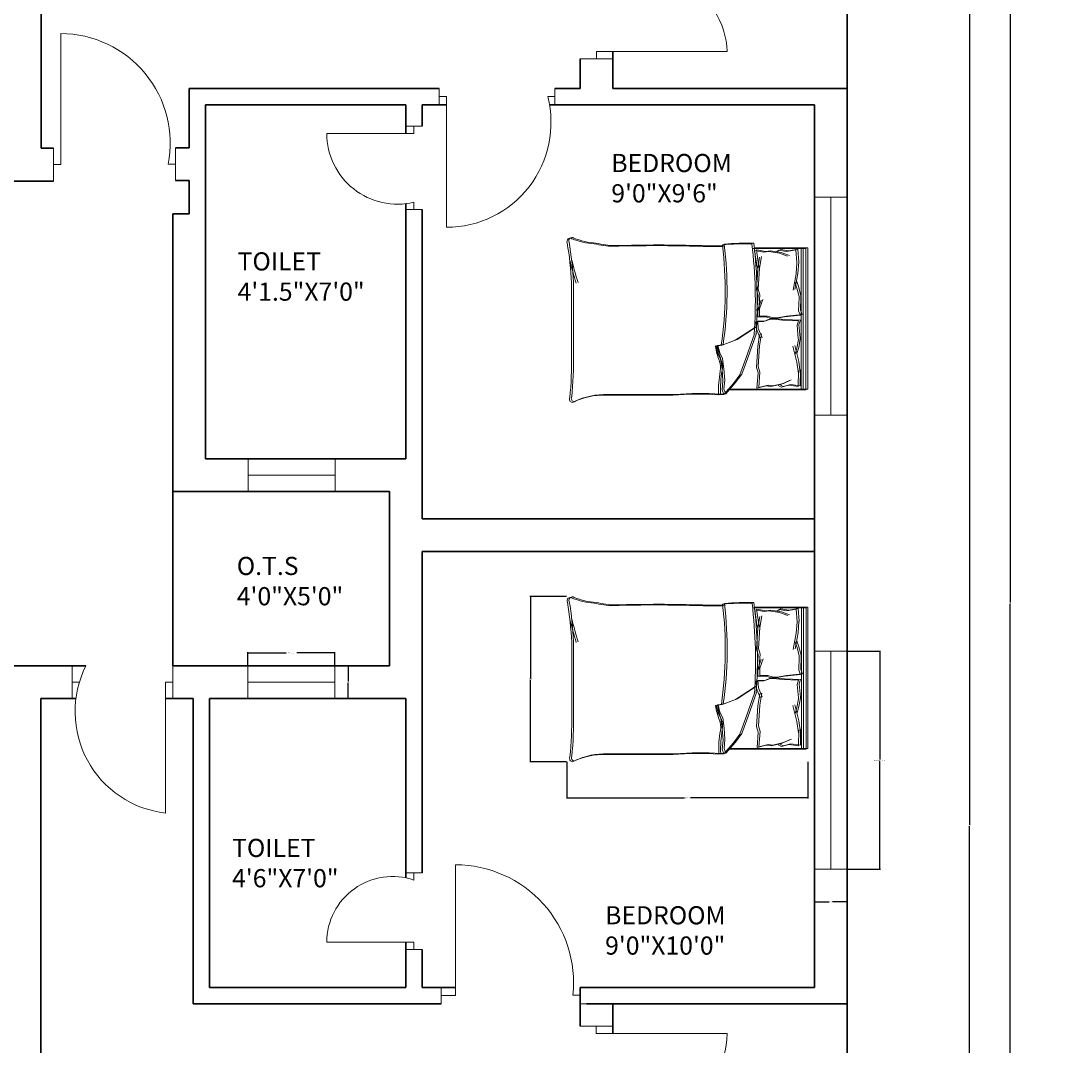
# Model space of a CAD drawing. Units: inches. Extents: x 2250 to 3629, y 982 to 2740.
# Tile 4 of 12: x 2629 to 2918, y 1543 to 1825. Entities that reach past the tile are written whole.
import ezdxf

# ---------------------------------------------------------------- set-up
doc = ezdxf.new("R2010")
doc.units = ezdxf.units.IN
for name, color, linetype, lineweight in [('A-ANNO-DIMS', 2, 'Continuous', 18), ('A-AREA-IDEN', 7, 'Continuous', 18), ('A-DOOR', 3, 'Continuous', 18), ('A-FURN', 8, 'Continuous', 13), ('A-GLAZ', 4, 'Continuous', 18), ('A-WALL', 7, 'Continuous', 35)]:
    doc.layers.add(name, color=color, linetype=linetype, lineweight=lineweight)
doc.styles.get("Standard").update_dxf_attribs({"font": 'arial.ttf'})
doc.dimstyles.get("Standard").update_dxf_attribs({"dimtxt": 0.18, "dimasz": 0.18, "dimexe": 0.18, "dimexo": 0.0625, "dimgap": 0.09, "dimtad": 0, "dimtih": 1, "dimtoh": 1, "dimdec": 4, "dimzin": 0, "dimdsep": 46, "dimtxsty": 'Standard', "dimcen": 0.09, "dimadec": 0, "dimazin": 0, "dimtfac": 1, "dimtdec": 4, "dimtofl": 0, "dimtmove": 0, "dimatfit": 3, "dimfxl": 1, "dimtolj": 1, "dimtzin": 0, "dimarcsym": 0})

# ---------------------------------------------------------------- blocks, each defined once
blk = doc.blocks.new('DR-36-BED-EAST-N')
for p, q in [((0, 38.25), (0, 33.75)), ((31.87, 33.75), (31.87, 38.25)), ((31.87, 38.25), (31.87, 36)), ((0, 33.75), (0, 36)), ((0, 36), (2, 36)), ((2, 36), (2, 0)), ((31.87, 36), (29.87, 36))]:
    blk.add_line(p, q)
blk.add_arc((2, 28.78), 28.78, 270, 14.5177)
blk = doc.blocks.new('DR-72-DECK-EAST-N')
for p, q in [((9, 42.6), (0, 42.6)), ((0, 42.6), (4.5, 42.6)), ((4.5, 42.6), (4.5, 40.6)), ((4.5, 40.6), (40.5, 40.6)), ((9, 0), (0, 0)), ((0, 0), (4.5, 0)), ((4.5, 0), (4.5, 2)), ((4.5, 2), (40.5, 2))]:
    blk.add_line(p, q)
for centre, radius, start, end in [((18.63, 40.6), 21.87, 295.9981, 0), ((18.59, 1.24), 21.93, 1.9829, 63.9515)]:
    blk.add_arc(centre, radius, start, end)
blk = doc.blocks.new('DR-36-BED-EAST-S')
for p, q in [((4, 2.25), (4, 38.25)), ((0, 4.5), (0, 0)), ((0, 0), (0, 2.25)), ((0, 2.25), (2, 2.25)), ((2, 2.25), (4, 2.25)), ((38.26, 2.37), (36.26, 2.37)), ((40.06, 0), (38.26, 0))]:
    blk.add_line(p, q)
blk.add_arc((4, 5.8), 32.45, 353.93, 90)
blk = doc.blocks.new('DR-72-DECK-EAST-S')
for p, q in [((5.33, 41.58), (0, 41.58)), ((0, 41.58), (4.45, 41.58)), ((9, 41.58), (1.67, 41.58)), ((1.67, 41.58), (5.33, 41.58)), ((4.45, 41.58), (4.45, 39.58)), ((4.45, 39.58), (40.45, 39.58)), ((4.5, 0), (4.5, 2)), ((4.5, 2), (40.5, 2)), ((9, 0), (0, 0)), ((0, 0), (4.5, 0))]:
    blk.add_line(p, q)
for centre, radius, start, end in [((18.64, 39.58), 21.82, 293.079, 0), ((16.02, -2.8), 24.94, 11.0871, 63.4091)]:
    blk.add_arc(centre, radius, start, end)
blk = doc.blocks.new('DR-24-BATH-EAST-S')
for p, q in [((21.75, 21.12), (26.25, 21.12)), ((26.25, 21.12), (24, 21.12)), ((24, 21.12), (24, 19.12)), ((24, 2), (0, 2)), ((24, 0), (24, 2)), ((26.25, 0), (21.75, 0)), ((21.75, 0), (24, 0))]:
    blk.add_line(p, q)
blk.add_arc((18.1, 2), 18.1, 70.988, 180)
blk = doc.blocks.new('DR-36-ENTRY-SE')
for p, q in [((0, 31.5), (0, 40.5)), ((27.72, 40.5), (27.72, 31.5)), ((0, 36), (2, 36)), ((27.72, 36), (25.72, 36)), ((25.72, 36), (25.72, 0)), ((27.72, 31.5), (27.72, 36))]:
    blk.add_line(p, q)
blk.add_arc((28.88, 27.9), 28.08, 153.3297, 263.5366)
blk = doc.blocks.new('DR-24-BATH-EAST-N')
for p, q in [((24, 20.95), (0, 20.95)), ((26.25, 22.95), (21.75, 22.95)), ((21.75, 22.95), (24, 22.95)), ((24, 22.95), (24, 20.95)), ((24, 0), (24, 2)), ((21.75, 0), (26.25, 0)), ((26.25, 0), (24, 0))]:
    blk.add_line(p, q)
blk.add_arc((19.48, 20.95), 19.48, 180, 283.4076)
blk = doc.blocks.new('DR-36-ENTRY-NE')
for p, q in [((2, 4.58), (2, 40.58)), ((0, 9), (0, 0)), ((33.56, 9.15), (33.56, 0.15)), ((0, 4.58), (2, 4.58)), ((33.56, 4.65), (31.56, 4.65))]:
    blk.add_line(p, q)
blk.add_arc((2, 10.45), 30.13, 348.9073, 90)
blk = doc.blocks.new('WIN-24-BATH-NW')
for p, q in [((9, 24), (0, 24)), ((0, 24), (4.5, 24)), ((4.5, 24), (4.5, 0)), ((9, 0), (0, 0)), ((4.5, 0), (9, 0))]:
    blk.add_line(p, q)
blk = doc.blocks.new('WIN-60-BED-EAST-S')
for p, q in [((0, 60), (9, 60)), ((9, 60), (4.5, 60)), ((4.5, 60), (4.5, 0)), ((9, 0), (0, 0)), ((4.5, 0), (9, 0))]:
    blk.add_line(p, q)
blk = doc.blocks.new('BED-WITH-PILLOWS')
for p, q in [((2.83, 51.56), (2.83, 66.3)), ((2.83, 66.3), (41.74, 66.3)), ((2.83, 65.05), (41.74, 65.05)), ((3.02, 51.04), (3.02, 65.78)), ((3.02, 65.78), (41.92, 65.78)), ((3.02, 64.53), (41.92, 64.53)), ((3.17, 63.59), (6.66, 63.85)), ((6.66, 63.85), (6.75, 63.84)), ((6.75, 63.84), (9.86, 63.6)), ((12.09, 63.25), (13.74, 63.84)), ((13.74, 63.84), (16.09, 64.43)), ((13.93, 63.32), (16.28, 63.91)), ((16.09, 64.43), (16.36, 64.43)), ((16.28, 63.91), (16.54, 63.91)), ((16.36, 64.43), (19.98, 64.31)), ((16.54, 63.91), (20.16, 63.79)), ((19.98, 64.31), (21.15, 64.78)), ((20.16, 63.79), (21.34, 64.26)), ((21.15, 64.78), (21.62, 60.43)), ((21.34, 64.26), (21.81, 59.9)), ((22.78, 64.27), (22.58, 59.9)), ((22.96, 63.75), (22.76, 59.38)), ((23.98, 63.88), (22.78, 64.27)), ((24.17, 63.36), (22.96, 63.75)), ((27.59, 64.22), (23.98, 63.88)), ((27.77, 63.7), (24.17, 63.36)), ((27.85, 64.24), (27.59, 64.22)), ((28.03, 63.72), (27.77, 63.7)), ((30.23, 63.8), (27.85, 64.24)), ((30.42, 63.28), (28.03, 63.72)), ((34.12, 63.8), (29.71, 62.7)), ((31.91, 63.31), (30.23, 63.8)), ((37.22, 64.23), (34.12, 63.8)), ((37.4, 63.71), (34.31, 63.28)), ((40.8, 64.22), (36.4, 64.3)), ((36.4, 64.3), (37.22, 64.23)), ((40.98, 63.7), (36.58, 63.78)), ((36.58, 63.78), (37.4, 63.71)), ((40.8, 64.22), (40.49, 61.61)), ((40.98, 63.7), (40.67, 61.09)), ((41.74, 66.3), (41.74, 44.64)), ((41.92, 65.78), (41.92, 44.12)), ((3.17, 63.6), (3.64, 61.01)), ((3.64, 61.01), (3.29, 58.89)), ((3.36, 63.06), (6.85, 63.33)), ((3.36, 63.08), (3.83, 60.49)), ((4.11, 59.01), (4.94, 61.25)), ((4.3, 58.49), (5.12, 60.73)), ((6.85, 63.33), (6.93, 63.32)), ((6.93, 63.32), (10.04, 63.08)), ((9.86, 63.6), (14.33, 62.78)), ((10.04, 63.08), (14.52, 62.26)), ((12.28, 62.73), (13.93, 63.32)), ((34.31, 63.28), (29.9, 62.18)), ((32.1, 62.79), (30.42, 63.28)), ((40.14, 59.58), (39.18, 61.76)), ((40.33, 59.06), (39.37, 61.24)), ((40.49, 61.61), (40.97, 59.51)), ((40.67, 61.09), (41.16, 58.99)), ((3.29, 58.89), (3.76, 58.07)), ((3.83, 60.49), (3.47, 58.37)), ((3.47, 58.37), (3.95, 57.55)), ((3.64, 56.07), (4.11, 59.01)), ((3.83, 55.55), (4.3, 58.49)), ((21.62, 60.43), (22.09, 57.84)), ((21.81, 59.9), (22.28, 57.32)), ((22.09, 57.84), (22.09, 56.78)), ((22.58, 59.9), (22.27, 57.28)), ((22.76, 59.38), (22.46, 56.76)), ((40.8, 56.67), (40.14, 59.58)), ((40.98, 56.15), (40.33, 59.06)), ((40.97, 59.51), (40.55, 58.66)), ((41.16, 58.99), (40.74, 58.14)), ((3.88, 54.78), (3.64, 56.07)), ((4.06, 54.25), (3.83, 55.55)), ((22.09, 56.78), (21.62, 55.25)), ((21.62, 55.25), (21.62, 53.06)), ((22.28, 56.26), (21.81, 54.73)), ((22.27, 57.28), (22.34, 56.23)), ((22.28, 57.32), (22.28, 56.26)), ((22.34, 56.23), (22.9, 54.73)), ((22.46, 56.76), (22.52, 55.71)), ((22.52, 55.71), (23.09, 54.21)), ((40.64, 55.37), (40.8, 56.67)), ((41.27, 52.81), (40.64, 55.37)), ((40.83, 54.85), (40.98, 56.15)), ((3.41, 52.19), (3.88, 54.78)), ((7.56, 52.77), (3.41, 52.19)), ((3.59, 51.66), (4.06, 54.25)), ((7.74, 52.25), (3.59, 51.66)), ((5.2, 53.58), (8.48, 53.04)), ((5.38, 53.06), (8.66, 52.52)), ((8.48, 53.04), (7.56, 52.77)), ((8.66, 52.52), (7.74, 52.25)), ((8.48, 53.04), (14.18, 52.69)), ((8.66, 52.52), (14.37, 52.17)), ((14.18, 52.69), (15.78, 53.14)), ((14.37, 52.17), (15.97, 52.62)), ((15.78, 53.14), (19.96, 52.81)), ((15.97, 52.62), (20.14, 52.29)), ((19.62, 53.06), (17.06, 53.95)), ((19.81, 52.54), (17.25, 53.43)), ((21.62, 53.06), (19.62, 53.06)), ((21.81, 52.54), (19.81, 52.54)), ((21.81, 54.73), (21.81, 52.54)), ((22.9, 54.73), (23.04, 52.55)), ((23.04, 52.55), (25.03, 52.68)), ((23.09, 54.21), (23.22, 52.03)), ((23.22, 52.03), (25.22, 52.15)), ((24.63, 52.15), (28.05, 46.86)), ((25.03, 52.68), (27.53, 53.72)), ((25.22, 52.15), (27.72, 53.2)), ((33.09, 49.76), (26.3, 52.15)), ((26.51, 53.58), (29.79, 53.04)), ((26.7, 53.06), (29.98, 52.52)), ((29.79, 53.04), (35.5, 52.69)), ((29.98, 52.52), (35.69, 52.17)), ((35.5, 52.69), (37.1, 53.14)), ((35.69, 52.17), (37.28, 52.62)), ((37.1, 53.14), (41.27, 52.81)), ((37.28, 52.62), (41.46, 52.29)), ((41.46, 52.29), (40.83, 54.85)), ((24.82, 51.63), (28.23, 46.34)), ((33.27, 49.24), (26.49, 51.63)), ((37.63, 48.12), (33.09, 49.76)), ((37.81, 47.6), (33.27, 49.24)), ((28.05, 46.86), (29.43, 43.21)), ((28.23, 46.34), (29.62, 42.69)), ((40.02, 46.36), (37.63, 48.12)), ((40.21, 45.84), (37.81, 47.6)), ((43.04, 43.71), (40.02, 46.36)), ((36.11, 43.21), (39.27, 43.46)), ((39.27, 43.46), (41.79, 43.21)), ((43.23, 43.19), (40.21, 45.84)), ((41.79, 43.21), (43.04, 43.71)), ((43.1, 42.29), (43.04, 43.71, 3.15)), ((29.43, 43.21), (29.68, 41.57)), ((29.62, 42.69), (29.87, 41.05)), ((29.68, 41.57), (31.7, 42.08)), ((29.87, 41.05), (31.89, 41.56)), ((31.7, 42.08), (33.34, 42.83)), ((31.89, 41.56), (33.53, 42.31)), ((33.34, 42.83), (36.11, 43.21)), ((33.53, 42.31), (36.3, 42.69)), ((36.3, 42.69), (39.45, 42.94)), ((39.45, 42.94), (41.97, 42.69)), ((41.97, 42.69), (43.23, 43.19)), ((43.29, 41.77), (43.23, 43.19, 3.15)), ((12.26, 1.79), (32.3, 1.79)), ((12.45, 1.27), (32.49, 1.27))]:
    blk.add_line(p, q)
for centre, radius, start, end in [((17.39, -81.91), 134.3, 86.0865, 96.7821), ((69.33, 49.94), 67.82, 178.7218, 185.604), ((69.52, 49.42), 67.82, 178.7218, 185.604), ((17.57, -82.43), 134.3, 86.0865, 96.7821), ((14.46, -60.96), 105.04, 81.7845, 96.9006), ((14.64, -61.48), 105.04, 81.7845, 96.9006), ((-136.21, 40.92), 138.49, 358.4762, 1.0082), ((-136.02, 40.4), 138.49, 358.4762, 1.0082), ((29.83, 41.52), 0.15, 160.2464, 271.1377), ((25.36, 65.1), 24.14, 280.6617, 289.8806), ((30.01, 41), 0.15, 160.2464, 271.1377), ((25.55, 64.58), 24.14, 280.6617, 289.8806), ((35.61, 37.76), 5.07, 78.6608, 113.7384), ((35.8, 37.23), 5.07, 78.6608, 113.7384), ((41.79, 71.72), 29.46, 259.8763, 272.5657), ((41.97, 71.2), 29.46, 259.8763, 272.5657), ((148.38, 36.74), 105.43, 176.9791, 183.8365), ((148.57, 36.22), 105.43, 176.9791, 183.8365), ((394.7, 25.1), 392.65, 178.2277, 181.7185), ((394.88, 24.58), 392.65, 178.2277, 181.7185), ((-3670.6, 11.09), 3713.84, 0.00217, 0.28689), ((-3670.41, 10.57), 3713.84, 0.00217, 0.28689), ((-21.9, 13.78), 24.13, 346.0648, 358.9113), ((-21.71, 13.26), 24.13, 346.0648, 358.9113), ((62, 10.4), 18.78, 177.4714, 206.4681), ((62.19, 9.88), 18.78, 177.4714, 206.4681), ((-17.63, 9.09), 19.18, 337.9751, 356.652), ((-17.45, 8.57), 19.18, 337.9751, 356.652), ((-14.02, 85.61), 86.67, 283.3832, 287.7053), ((0.89, 1.4), 0.887, 146.1736, 293.4781), ((1.07, 0.88), 0.887, 146.1736, 293.4781), ((17.44, -97.2), 99.12, 92.9958, 99.4091), ((17.63, -97.72), 99.12, 92.9958, 99.4091), ((-13.83, 85.09), 86.67, 283.3832, 287.7053), ((33.5, -106.51), 108.31, 84.4998, 90.6351), ((33.69, -107.03), 108.31, 84.4998, 90.6351), ((44.3, 2.09), 0.897, 242.6588, 356.02), ((44.48, 1.57), 0.897, 242.6588, 356.02)]:
    blk.add_arc(centre, radius, start, end)
blk = doc.blocks.new('*D57')
at = {"layer": 'A-ANNO-DIMS', "color": 0, "lineweight": -2, "transparency": 16777216}
for p, q in [((2779.45, 1620.81), (2779.45, 1610.74)), ((2845.84, 1620.81), (2845.84, 1610.74)), ((2779.63, 1610.92), (2811.82, 1610.92)), ((2845.66, 1610.92), (2813.46, 1610.92))]:
    blk.add_line(p, q, dxfattribs=at)
at = {"layer": 'A-ANNO-DIMS', "color": 0, "transparency": 16777216}
for points in [[(2779.63, 1610.95), (2779.63, 1610.89), (2779.45, 1610.92)], [(2845.66, 1610.95), (2845.66, 1610.89), (2845.84, 1610.92)]]:
    blk.add_solid(points, dxfattribs=at)
at = {"layer": 'Defpoints', "color": 0, "transparency": 16777216}
for p in [(2779.45, 1620.88), (2845.84, 1620.88), (2845.84, 1610.92)]:
    blk.add_point(p, dxfattribs=at)
at = {"layer": 'A-ANNO-DIMS', "color": 0, "transparency": 16777216, "insert": (2812.64, 1610.92), "char_height": 0.18, "attachment_point": 5}
blk.add_mtext('\\A1;BED 66 TYP.', dxfattribs=at)
blk = doc.blocks.new('*D58')
at = {"layer": 'A-ANNO-DIMS', "color": 0, "lineweight": -2, "transparency": 16777216}
for p, q in [((2779.38, 1666.32), (2769.31, 1666.32)), ((2769.49, 1666.14), (2769.49, 1643.78)), ((2769.49, 1621.06), (2769.49, 1643.42)), ((2779.38, 1620.88), (2769.31, 1620.88))]:
    blk.add_line(p, q, dxfattribs=at)
at = {"layer": 'A-ANNO-DIMS', "color": 0, "transparency": 16777216}
for points in [[(2769.46, 1666.14), (2769.52, 1666.14), (2769.49, 1666.32)], [(2769.46, 1621.06), (2769.52, 1621.06), (2769.49, 1620.88)]]:
    blk.add_solid(points, dxfattribs=at)
at = {"layer": 'Defpoints', "color": 0, "transparency": 16777216}
for p in [(2779.45, 1666.32), (2769.49, 1620.88), (2779.45, 1620.88)]:
    blk.add_point(p, dxfattribs=at)
at = {"layer": 'A-ANNO-DIMS', "color": 0, "transparency": 16777216, "insert": (2769.49, 1643.6), "char_height": 0.18, "attachment_point": 5}
blk.add_mtext('\\A1;45 TYP.', dxfattribs=at)
blk = doc.blocks.new('*D73')
at = {"layer": 'A-ANNO-DIMS', "color": 0, "lineweight": -2, "transparency": 16777216}
for p, q in [((2691.61, 1647.29), (2691.61, 1651.01)), ((2715.61, 1647.31), (2715.61, 1651.02)), ((2691.79, 1650.83), (2702.13, 1650.83)), ((2715.43, 1650.84), (2705.09, 1650.84))]:
    blk.add_line(p, q, dxfattribs=at)
at = {"layer": 'A-ANNO-DIMS', "color": 0, "transparency": 16777216}
for points in [[(2715.43, 1650.87), (2715.43, 1650.81), (2715.61, 1650.84)], [(2691.79, 1650.86), (2691.79, 1650.8), (2691.61, 1650.83)]]:
    blk.add_solid(points, dxfattribs=at)
at = {"layer": 'Defpoints', "color": 0, "transparency": 16777216}
for p in [(2691.61, 1650.83), (2691.61, 1647.23), (2715.61, 1647.24)]:
    blk.add_point(p, dxfattribs=at)
at = {"layer": 'A-ANNO-DIMS', "color": 0, "transparency": 16777216, "insert": (2703.61, 1650.84), "char_height": 0.18, "attachment_point": 5}
blk.add_mtext('\\A1;BATH WINDOW 24 TYP.', dxfattribs=at)
blk = doc.blocks.new('*D74')
at = {"layer": 'A-ANNO-DIMS', "color": 0, "lineweight": -2, "transparency": 16777216}
for p, q in [((2715.67, 1647.24), (2719.39, 1647.25)), ((2719.21, 1647.07), (2719.21, 1642.93)), ((2719.22, 1638.43), (2719.21, 1642.57)), ((2715.68, 1638.24), (2719.4, 1638.25))]:
    blk.add_line(p, q, dxfattribs=at)
at = {"layer": 'A-ANNO-DIMS', "color": 0, "transparency": 16777216}
for points in [[(2719.24, 1647.07), (2719.18, 1647.07), (2719.21, 1647.25)], [(2719.25, 1638.43), (2719.19, 1638.43), (2719.22, 1638.25)]]:
    blk.add_solid(points, dxfattribs=at)
at = {"layer": 'Defpoints', "color": 0, "transparency": 16777216}
for p in [(2715.61, 1647.24), (2719.21, 1647.25), (2715.62, 1638.24)]:
    blk.add_point(p, dxfattribs=at)
at = {"layer": 'A-ANNO-DIMS', "color": 0, "transparency": 16777216, "insert": (2719.21, 1642.75), "char_height": 0.18, "attachment_point": 5}
blk.add_mtext('\\A1;9 TYP.', dxfattribs=at)
blk = doc.blocks.new('*D79')
at = {"layer": 'A-ANNO-DIMS', "color": 0, "lineweight": -2, "transparency": 16777216}
for p, q in [((2856.67, 1651.29), (2865.79, 1651.29)), ((2865.61, 1651.11), (2865.61, 1621.47)), ((2865.61, 1591.47), (2865.61, 1621.11)), ((2856.67, 1591.29), (2865.79, 1591.29))]:
    blk.add_line(p, q, dxfattribs=at)
at = {"layer": 'A-ANNO-DIMS', "color": 0, "transparency": 16777216}
for points in [[(2865.58, 1651.11), (2865.64, 1651.11), (2865.61, 1651.29)], [(2865.58, 1591.47), (2865.64, 1591.47), (2865.61, 1591.29)]]:
    blk.add_solid(points, dxfattribs=at)
at = {"layer": 'Defpoints', "color": 0, "transparency": 16777216}
for p in [(2856.61, 1651.29), (2865.61, 1651.29), (2856.61, 1591.29)]:
    blk.add_point(p, dxfattribs=at)
at = {"layer": 'A-ANNO-DIMS', "color": 0, "transparency": 16777216, "insert": (2865.61, 1621.29), "char_height": 0.18, "attachment_point": 5}
blk.add_mtext('\\A1;BEDROOM WINDOW 60 TYP.', dxfattribs=at)
blk = doc.blocks.new('*D80')
at = {"layer": 'A-ANNO-DIMS', "color": 0, "lineweight": -2, "transparency": 16777216}
for p, q in [((2847.61, 1591.23), (2847.61, 1582.11)), ((2856.61, 1591.23), (2856.61, 1582.11)), ((2847.79, 1582.29), (2851.65, 1582.29)), ((2856.43, 1582.29), (2852.57, 1582.29))]:
    blk.add_line(p, q, dxfattribs=at)
at = {"layer": 'A-ANNO-DIMS', "color": 0, "transparency": 16777216}
for points in [[(2847.79, 1582.32), (2847.79, 1582.26), (2847.61, 1582.29)], [(2856.43, 1582.32), (2856.43, 1582.26), (2856.61, 1582.29)]]:
    blk.add_solid(points, dxfattribs=at)
at = {"layer": 'Defpoints', "color": 0, "transparency": 16777216}
for p in [(2847.61, 1591.29), (2856.61, 1591.29), (2856.61, 1582.29)]:
    blk.add_point(p, dxfattribs=at)
at = {"layer": 'A-ANNO-DIMS', "color": 0, "transparency": 16777216, "insert": (2852.11, 1582.29), "char_height": 0.18, "attachment_point": 5}
blk.add_mtext('\\A1;9 TYP.', dxfattribs=at)
blk = doc.blocks.new('*D170')
at = {"layer": 'A-ANNO-DIMS', "color": 0, "lineweight": -2, "transparency": 16777216}
for p, q in [((2855.4, 2070.24), (2901.69, 2070.24)), ((2901.51, 2070.06), (2901.51, 1664.67)), ((2901.51, 1258.92), (2901.51, 1664.3)), ((2481.67, 1258.74), (2901.69, 1258.74))]:
    blk.add_line(p, q, dxfattribs=at)
at = {"layer": 'A-ANNO-DIMS', "color": 0, "transparency": 16777216}
for points in [[(2901.48, 2070.06), (2901.54, 2070.06), (2901.51, 2070.24)], [(2901.48, 1258.92), (2901.54, 1258.92), (2901.51, 1258.74)]]:
    blk.add_solid(points, dxfattribs=at)
at = {"layer": 'Defpoints', "color": 0, "transparency": 16777216}
for p in [(2855.34, 2070.24), (2901.51, 2070.24), (2481.61, 1258.74)]:
    blk.add_point(p, dxfattribs=at)
at = {"layer": 'A-ANNO-DIMS', "color": 0, "transparency": 16777216, "insert": (2901.51, 1664.49), "char_height": 0.18, "attachment_point": 5}
blk.add_mtext('\\A1;811.5', dxfattribs=at)
blk = doc.blocks.new('*D173')
at = {"layer": 'A-ANNO-DIMS', "color": 0, "lineweight": -2, "transparency": 16777216}
for p, q in [((2932.01, 1947.92), (2890.14, 1947.92)), ((2890.32, 1947.74), (2890.32, 1603.51)), ((2890.32, 1258.92), (2890.32, 1603.15)), ((2981.16, 1258.74), (2890.14, 1258.74))]:
    blk.add_line(p, q, dxfattribs=at)
at = {"layer": 'A-ANNO-DIMS', "color": 0, "transparency": 16777216}
for points in [[(2890.29, 1947.74), (2890.35, 1947.74), (2890.32, 1947.92)], [(2890.29, 1258.92), (2890.35, 1258.92), (2890.32, 1258.74)]]:
    blk.add_solid(points, dxfattribs=at)
at = {"layer": 'Defpoints', "color": 0, "transparency": 16777216}
for p in [(2932.07, 1947.92), (2890.32, 1258.74), (2981.23, 1258.74)]:
    blk.add_point(p, dxfattribs=at)
at = {"layer": 'A-ANNO-DIMS', "color": 0, "transparency": 16777216, "insert": (2890.32, 1603.33), "char_height": 0.18, "attachment_point": 5}
blk.add_mtext('\\A1;689.2', dxfattribs=at)

msp = doc.modelspace()

# ---------------------------------------------------------------- linework, layer by layer
at = {"layer": 'A-WALL'}
for p, q in [((2856.6072, 2029.7354), (2856.6072, 1276.7354)), ((2634.7014, 1926.2354), (2634.7014, 1789.7354)), ((2792.1072, 1806.2354), (2792.1072, 1816.3801)), ((2783.1072, 1814.3801), (2783.1072, 1806.2354)), ((2675.4769, 1806.2354), (2735.1072, 1806.2354)), ((2675.4769, 1789.8862), (2675.4769, 1806.2354)), ((2744.3192, 1806.2354), (2735.1072, 1806.2354)), ((2783.1072, 1806.2354), (2776.1844, 1806.2354)), ((2792.1072, 1806.2354), (2856.6072, 1806.2354)), ((2675.4769, 1801.7354), (2675.4769, 1789.8862)), ((2735.1072, 1801.7354), (2679.9769, 1801.7354)), ((2679.9769, 1704.2354), (2679.9769, 1801.7354)), ((2735.1072, 1801.7354), (2735.1072, 1793.8422)), ((2739.6072, 1801.7354), (2739.6072, 1795.8422)), ((2746.3192, 1801.7354), (2739.6072, 1801.7354)), ((2847.6072, 1801.7354), (2774.672, 1801.7354)), ((2783.1072, 1801.7354), (2847.6072, 1801.7354)), ((2783.1072, 1801.7354), (2792.1072, 1801.7354)), ((2847.6072, 1801.7354), (2847.6072, 1558.7354)), ((2634.7014, 1789.7354), (2638.1007, 1789.7354)), ((2675.4769, 1789.8862), (2671.6658, 1789.8862)), ((2634.7014, 1780.7354), (2625.6072, 1780.7354)), ((2638.1007, 1780.7354), (2634.7014, 1780.7354)), ((2671.6658, 1780.8862), (2675.4769, 1780.8862)), ((2675.4769, 1771.6808), (2675.4769, 1780.8862)), ((2675.4769, 1780.8862), (2675.4769, 1771.6808)), ((2735.1072, 1774.4922), (2735.1072, 1704.2354)), ((2739.6072, 1772.8908), (2739.6072, 1687.7354)), ((2670.9769, 1704.2354), (2670.9769, 1771.6808)), ((2670.9769, 1771.6808), (2675.4769, 1771.6808)), ((2670.9769, 1647.2354), (2670.9769, 1704.2354)), ((2679.9769, 1704.2354), (2735.1072, 1704.2354)), ((2730.6072, 1695.2354), (2670.9769, 1695.2354)), ((2730.6072, 1647.2354), (2730.6072, 1695.2354)), ((2739.6072, 1687.7354), (2783.1072, 1687.7354)), ((2783.1072, 1687.7354), (2847.6072, 1687.7354)), ((2783.1072, 1678.7354), (2739.6072, 1678.7354)), ((2739.6072, 1678.7354), (2739.6072, 1590.2852)), ((2783.1072, 1678.7354), (2847.6072, 1678.7354)), ((2647.0484, 1647.2354), (2622.9956, 1647.2354)), ((2676.6072, 1647.2354), (2670.9769, 1647.2354)), ((2726.1072, 1647.2354), (2676.6072, 1647.2354)), ((2726.1072, 1647.2354), (2730.6072, 1647.2354)), ((2634.6072, 1638.2354), (2634.6072, 1434.2354)), ((2634.6072, 1638.2354), (2644.2932, 1638.2354)), ((2668.9769, 1638.2354), (2676.6072, 1638.2354)), ((2676.6072, 1638.2354), (2676.6072, 1554.2354)), ((2681.1072, 1558.7354), (2681.1072, 1638.2354)), ((2681.1072, 1638.2354), (2735.1072, 1638.2354)), ((2735.1072, 1638.2354), (2735.1072, 1588.9015)), ((2735.1072, 1638.2354), (2735.1072, 1588.9015)), ((2735.1072, 1571.1699), (2735.1072, 1558.7354)), ((2735.1072, 1571.1699), (2735.1072, 1558.7354)), ((2739.6072, 1569.1699), (2739.6072, 1558.7354)), ((2676.6072, 1554.2354), (2676.6072, 1558.7354)), ((2681.1072, 1558.7354), (2735.1072, 1558.7354)), ((2739.6072, 1558.7354), (2748.8426, 1558.7354)), ((2783.1072, 1558.7354), (2847.6072, 1558.7354)), ((2783.1072, 1548.0588), (2783.1072, 1558.7354)), ((2676.6072, 1554.2354), (2681.1072, 1554.2354)), ((2681.1072, 1554.2354), (2676.6072, 1554.2354)), ((2735.1072, 1554.2354), (2681.1072, 1554.2354)), ((2735.1072, 1554.2354), (2744.8426, 1554.2354)), ((2784.9057, 1554.2354), (2847.6072, 1554.2354)), ((2856.6072, 1554.2354), (2787.6072, 1554.2354)), ((2792.1072, 1546.0588), (2792.1072, 1554.2354))]:
    msp.add_line(p, q, dxfattribs=at)

# ---------------------------------------------------------------- block references
at = {"layer": 'A-DOOR'}
for name, p in [('DR-72-DECK-EAST-N', (2783.107, 1814.38)), ('DR-36-ENTRY-NE', (2638.101, 1780.735)), ('DR-36-BED-EAST-N', (2744.319, 1767.985)), ('DR-24-BATH-EAST-N', (2713.357, 1772.891)), ('DR-36-ENTRY-SE', (2643.256, 1606.735)), ('DR-24-BATH-EAST-S', (2713.357, 1569.17)), ('DR-36-BED-EAST-S', (2744.843, 1554.235)), ('DR-72-DECK-EAST-S', (2783.107, 1506.481))]:
    msp.add_blockref(name, p, dxfattribs=at)
at = {"layer": 'A-FURN', "rotation": 270.0000000000001}
for p in [(2779.4898, 1765.1768), (2779.5333, 1666.2532)]:
    msp.add_blockref('BED-WITH-PILLOWS', p, dxfattribs=at)
at = {"layer": 'A-GLAZ'}
for p in [(2847.607, 1716.2735), (2847.607, 1591.289)]:
    msp.add_blockref('WIN-60-BED-EAST-S', p, dxfattribs=at)
for p, rotation in [((2715.6631, 1695.2352), 89.99999999999808), ((2715.6174, 1638.2448), 90.04567875527589)]:
    msp.add_blockref('WIN-24-BATH-NW', p, dxfattribs=dict(at, rotation=rotation))

# ---------------------------------------------------------------- texts
at = {"layer": 'A-AREA-IDEN', "char_height": 5, "attachment_point": 1}
for s, width, insert in [('BEDROOM\\P9\'0"X9\'6"', 121.232209, (2791.7003, 1788.1912)), ('TOILET\\P4\'1.5"X7\'0"', 106.246248, (2688.7914, 1761.1133)), ('O.T.S\\P4\'0"X5\'0"', 89.276977, (2688.575, 1677.2676)), ('TOILET\\P4\'6"X7\'0"', 97.949394, (2687.2798, 1599.636)), ('BEDROOM\\P9\'0"X10\'0"', 104.379349, (2790.0005, 1581.0925))]:
    msp.add_mtext_dynamic_manual_height_columns(s, width=width, gutter_width=12.5, heights=[0], dxfattribs=dict(at, insert=insert))

# ---------------------------------------------------------------- dimensions: what is measured, and where the dimension line sits
at = {"layer": 'A-ANNO-DIMS'}
for base, p1, p2, picture, middle in [((2901.5072, 2070.2354), (2481.6072, 1258.7354), (2855.3384, 2070.2354), '*D170', (2901.5072, 1664.4854)), ((2890.3241, 1258.7354), (2932.0741, 1947.9231), (2981.2267, 1258.7354), '*D173', (2890.3241, 1603.3293))]:
    dim = msp.add_linear_dim(base=base, p1=p1, p2=p2, angle=90, dimstyle='Standard', override={"dimdec": 1, "dimlfac": 1, "dimrnd": 0, "dimzin": 0, "dimdsep": 46, "dimlunit": 2}, dxfattribs=at)
    dim.commit()
    dim.dimension.update_dxf_attribs({"geometry": picture, "text_midpoint": middle})
for base, p1, p2, angle, text, picture, middle in [((2769.4886, 1620.8763), (2779.447, 1666.3232), (2779.447, 1620.8763), 270, '<> TYP.', '*D58', (2769.4886, 1643.5997)), ((2691.6079, 1650.8259), (2715.6107, 1647.245), (2691.6107, 1647.2259), 180.045679, 'BATH WINDOW <> TYP.', '*D73', (2703.6078, 1650.8354)), ((2865.6072, 1651.2895), (2856.6072, 1591.2895), (2856.6072, 1651.2895), 90, 'BEDROOM WINDOW <> TYP.', '*D79', (2865.6072, 1621.2895)), ((2719.2107, 1647.2479), (2715.6179, 1638.245), (2715.6107, 1647.245), 90.045679, '<> TYP.', '*D74', (2719.2143, 1642.7479)), ((2845.8362, 1610.9179), (2779.447, 1620.8763), (2845.8362, 1620.8763), 0, 'BED <> TYP.', '*D57', (2812.6416, 1610.9179))]:
    dim = msp.add_linear_dim(base=base, p1=p1, p2=p2, angle=angle, text=text, dimstyle='Standard', override={"dimdec": 0, "dimlfac": 1, "dimrnd": 0, "dimzin": 0, "dimdsep": 46, "dimlunit": 2}, dxfattribs=at)
    dim.commit()
    dim.dimension.update_dxf_attribs({"geometry": picture, "text_midpoint": middle})
dim = msp.add_linear_dim(base=(2856.6072, 1582.2895), p1=(2847.6072, 1591.2895), p2=(2856.6072, 1591.2895), text='<> TYP.', dimstyle='Standard', override={"dimdec": 0, "dimlfac": 1, "dimrnd": 0, "dimzin": 0, "dimdsep": 46, "dimlunit": 2}, dxfattribs=at)
dim.commit()
dim.dimension.update_dxf_attribs({"geometry": '*D80', "text_midpoint": (2852.1072, 1582.2895)})

doc.saveas('drawing.dxf')
